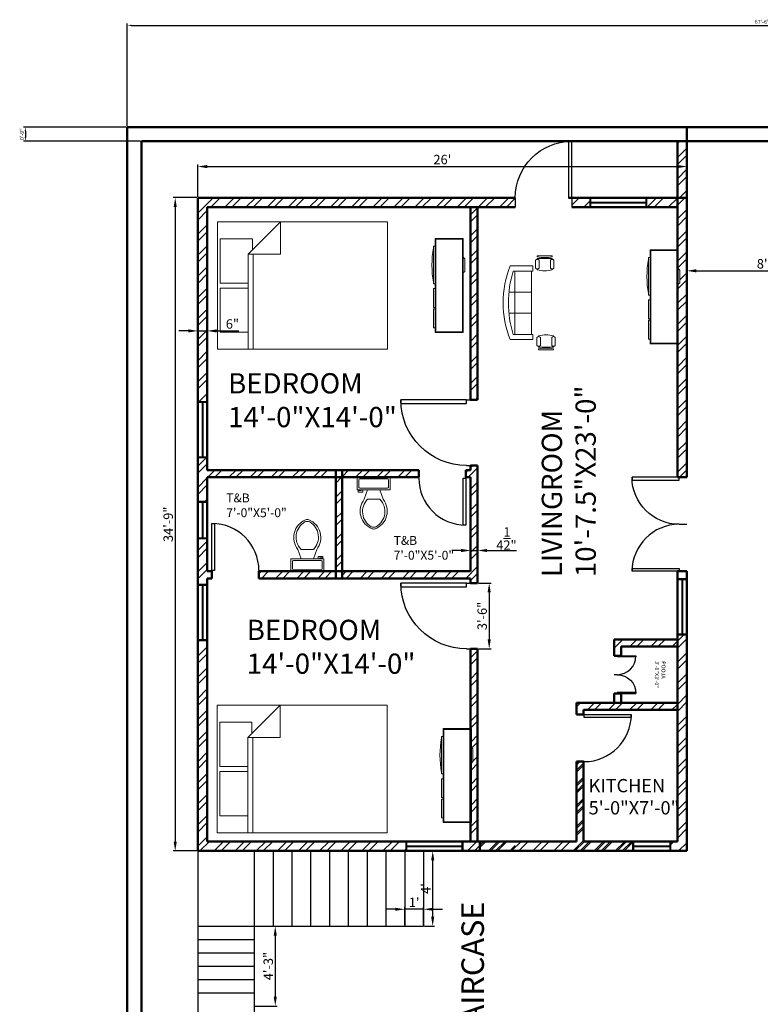
# Model space of a CAD drawing. Units: inches. Extents: x -12550 to 6516, y 1273 to 18700.
# Tile 18 of 19: x 5571 to 6043, y 1958 to 2587. Entities that reach past the tile are written whole.
import ezdxf

# ---------------------------------------------------------------- set-up
doc = ezdxf.new("R2010")
doc.units = ezdxf.units.IN
for name, color, linetype, lineweight in [('A-ANNO-DIMS', 2, 'Continuous', 18), ('A-AREA-IDEN', 1, 'Continuous', 18), ('A-DOOR', 5, 'Continuous', 25), ('A-FLOR-STRS', 6, 'Continuous', 25), ('A-FURN', 8, 'Continuous', 18), ('A-GLAZ', 3, 'Continuous', 25), ('A-WALL', 7, 'Continuous', 50), ('A-WALL-PATT', 8, 'Continuous', 13)]:
    doc.layers.add(name, color=color, linetype=linetype, lineweight=lineweight)
doc.styles.get("Standard").update_dxf_attribs({"font": 'arial.ttf'})
doc.dimstyles.new('ISO-25', dxfattribs={"dimtxt": 2.5, "dimasz": 2.5, "dimexe": 1.25, "dimexo": 0.625, "dimtad": 1, "dimlunit": 4, "dimtxsty": 'Standard', "dimcen": 2.5, "dimadec": 0, "dimazin": 0, "dimtfac": 1, "dimtmove": 0, "dimatfit": 3, "dimfxl": 1, "dimarcsym": 0})
pattern_1 = [(45, (3666.851, 0), (-6.735192, 6.735192), []), (45, (3671.341, 0), (-6.735192, 6.735192), [])]
pattern_2 = [(45, (3666.851, 567), (-6.735192, 6.735192), []), (45, (3671.341, 567), (-6.735192, 6.735192), [])]

# ---------------------------------------------------------------- blocks, each defined once
blk = doc.blocks.new('*U2')
for p, q in [((0, 0), (0, -5)), ((30, 0), (30, -5))]:
    blk.add_line(p, q)
blk.add_lwpolyline([(0, 0), (0, 30), (1.75, 30), (1.75, 0)], close=True)
blk.add_arc((0, 0), 30, 0, 90)
blk = doc.blocks.new('Bed - Queen')
for p, q in [((0, -80.00003), (0, 0)), ((0, 0), (59.99999, 0)), ((59.99999, 0), (59.99999, -80.00003)), ((7.99999, -1.2), (28.79998, -1.2)), ((7.99999, -14.4), (7.99999, -1.2)), ((28.79998, -1.2), (28.79998, -14.4)), ((31.19999, -1.2), (51.99999, -1.2)), ((31.19999, -14.4), (31.19999, -1.2)), ((51.99999, -1.2), (51.99999, -16.4)), ((0, -14.4), (44.8, -14.4)), ((44.8, -16.8), (0, -16.8)), ((59.99999, -29.6), (44.8, -14.4)), ((44.8, -14.4), (44.8, -29.6)), ((51.99999, -16.4), (46.79936, -16.4)), ((44.8, -29.6), (59.99999, -29.6)), ((59.99999, -80.00003), (0, -80.00003))]:
    blk.add_line(p, q)
blk = doc.blocks.new('Toilet - top')
for p, q in [((9.5, -6), (9.5, -2)), ((-10, -8.5), (-8, -8.5)), ((-10, -9.5), (-10, -8.5)), ((-7, -9.5), (-10, -9.5)), ((-8, -8.5), (-8, -8)), ((-7, -8), (-7, -9.5)), ((-4, -8), (-6, -14)), ((4, -8), (6, -14)), ((4, -14), (-4, -14))]:
    blk.add_line(p, q)
blk.add_lwpolyline([(10.5, -8), (10.5, 0), (-10.5, 0), (-10.5, -8)], close=True)
for points in [[(-9.5, -2), (-9.5, -6)], [(8.5, -1), (-8.5, -1)], [(-8.5, -7), (8.5, -7)]]:
    blk.add_lwpolyline(points)
for centre, radius, start, end in [((-8.62, -1.88), 0.884, 81.8699, 188.1301), ((-8.62, -6.12), 0.884, 171.8699, 278.1301), ((8.62, -1.88), 0.884, 351.8699, 98.1301), ((8.62, -6.12), 0.884, 261.8699, 8.1301), ((3.52, -21.58), 12.17, 141.46911, 247.97143), ((4.2, -21.82), 11.33, 136.36773, 238.94682), ((-3.52, -21.58), 12.17, 292.02843, 38.53071), ((-4.2, -21.82), 11.33, 301.05301, 43.63209), ((0, -27.88), 4, 245.73182, 294.26817), ((0, -29), 4, 254.86053, 285.13947)]:
    blk.add_arc(centre, radius, start, end)
blk = doc.blocks.new('Entertainment Center')
for p, q in [((-4, 0), (-5, -1)), ((4, 0), (-4, 0)), ((5, -1), (4, 0)), ((-17, -19), (-17, -1)), ((-17, -1), (43, -1)), ((-16.5, -18.5), (-16.5, -1.5)), ((-16.5, -1.5), (42.5, -1.5)), ((42.5, -1.5), (42.5, -18.5)), ((43, -1), (43, -19)), ((42.5, -18.5), (-16.5, -18.5)), ((43, -19), (-17, -19)), ((-12, -20), (-12, -19)), ((12, -20), (-12, -20)), ((12, -19), (12, -20)), ((15, -20), (15, -19)), ((27, -20), (15, -20)), ((27, -19), (27, -20)), ((28, -20), (28, -19)), ((40, -20), (28, -20)), ((40, -19), (40, -20))]:
    blk.add_line(p, q)
blk.add_arc((0, 40), 61, 259.6111, 280.3889)
blk = doc.blocks.new('Sofa - Roundback 7 ft.')
for p, q in [((-12.00002, -32.4421), (-12.00003, -6.5971)), ((11.99997, -32.4421), (11.99998, -6.5971)), ((-36.000027, -34), (-36.000027, -11.4696)), ((-35.999844, -13.3819), (35.9998, -13.3819)), ((35.99998, -34), (35.99998, -11.4696)), ((-36.000027, -32.4421), (35.99998, -32.4421))]:
    blk.add_line(p, q)
for points in [[(-36.000027, -34), (-42.000027, -34), (-42.000027, -8)], [(41.99998, -8), (41.99998, -34), (35.99998, -34)]]:
    blk.add_lwpolyline(points)
for centre, radius, start, end in [((0, -114.25), 114.25, 68.43141, 111.5686), ((-0.00001, -127.1968), 121.1968, 72.72033, 107.2797)]:
    blk.add_arc(centre, radius, start, end)
blk = doc.blocks.new('Chair - Desk')
for p, q in [((-8.5, 0), (-8.5, -1)), ((-8.5, 0), (8.5, 0)), ((8.5, 0), (8.5, -1)), ((-10.5, -5), (-10.5, -14)), ((-8.5, -3), (-8.5, -4)), ((-8.5, -3), (8.5, -3)), ((-6.5, -14), (-6.5, -5)), ((-2, -3), (-2, -1.9355)), ((2, -1.9576), (2, -3)), ((6.5, -5), (6.5, -14)), ((8.5, -3), (8.5, -4)), ((10.5, -14), (10.5, -5)), ((-8.5, -15), (-8.5, -16)), ((8.5, -15), (8.5, -16))]:
    blk.add_line(p, q)
for centre, radius, start, end in [((-8.5, -6.5), 2.5, 36.8699, 143.1301), ((0, 34.625), 36.625, 256.5803, 283.4197), ((8.5, -6.5), 2.5, 36.8699, 143.1301), ((-8.5, -12.5), 2.5, 216.8699, 323.1301), ((0, 19.625), 36.625, 256.5803, 283.4197), ((8.5, -12.5), 2.5, 216.8699, 323.1301)]:
    blk.add_arc(centre, radius, start, end)
blk = doc.blocks.new('*D49')
at = {"layer": 'A-ANNO-DIMS', "color": 0, "lineweight": -2, "transparency": 16777216}
for p, q in [((5684.54, 2388.03), (5684.54, 2389.43)), ((5690.54, 2388.03), (5690.54, 2389.43)), ((5678.54, 2388.18), (5672.54, 2388.18)), ((5684.54, 2388.18), (5690.54, 2388.18)), ((5696.54, 2388.18), (5710.72, 2388.18))]:
    blk.add_line(p, q, dxfattribs=at)
at = {"layer": 'A-ANNO-DIMS', "color": 0, "transparency": 16777216}
for points in [[(5678.54, 2389.18), (5678.54, 2387.18), (5684.54, 2388.18)], [(5696.54, 2389.18), (5696.54, 2387.18), (5690.54, 2388.18)]]:
    blk.add_solid(points, dxfattribs=at)
at = {"layer": 'Defpoints', "color": 0, "transparency": 16777216}
for p in [(5684.54, 2387.4), (5690.54, 2388.18), (5690.54, 2387.4)]:
    blk.add_point(p, dxfattribs=at)
at = {"layer": 'A-ANNO-DIMS', "color": 0, "transparency": 16777216, "insert": (5706.63, 2391.87), "char_height": 6, "attachment_point": 5}
blk.add_mtext('6"', dxfattribs=at)
blk = doc.blocks.new('*D50')
at = {"layer": 'A-ANNO-DIMS', "color": 0, "lineweight": -2, "transparency": 16777216}
for p, q in [((5858.54, 2251.78), (5858.54, 2246.78)), ((5863.04, 2251.78), (5863.04, 2246.78)), ((5852.54, 2248.03), (5846.54, 2248.03)), ((5858.54, 2248.03), (5863.04, 2248.03)), ((5869.04, 2248.03), (5887.8, 2248.03))]:
    blk.add_line(p, q, dxfattribs=at)
at = {"layer": 'A-ANNO-DIMS', "color": 0, "transparency": 16777216}
for points in [[(5852.54, 2249.03), (5852.54, 2247.03), (5858.54, 2248.03)], [(5869.04, 2249.03), (5869.04, 2247.03), (5863.04, 2248.03)]]:
    blk.add_solid(points, dxfattribs=at)
at = {"layer": 'Defpoints', "color": 0, "transparency": 16777216}
for p in [(5858.54, 2252.41), (5863.04, 2252.41), (5863.04, 2248.03)]:
    blk.add_point(p, dxfattribs=at)
at = {"layer": 'A-ANNO-DIMS', "color": 0, "transparency": 16777216, "insert": (5881.42, 2255.68), "char_height": 6, "attachment_point": 5}
blk.add_mtext('4{\\H1x;\\S1/2;}"', dxfattribs=at)
blk = doc.blocks.new('*D57')
at = {"layer": 'A-ANNO-DIMS', "color": 0, "lineweight": -2, "transparency": 16777216}
for p, q in [((5863.66, 2227.25), (5871.67, 2227.25)), ((5870.42, 2221.25), (5870.42, 2191.25)), ((5863.66, 2185.25), (5871.67, 2185.25))]:
    blk.add_line(p, q, dxfattribs=at)
at = {"layer": 'A-ANNO-DIMS', "color": 0, "transparency": 16777216}
for points in [[(5869.42, 2221.25), (5871.42, 2221.25), (5870.42, 2227.25)], [(5869.42, 2191.25), (5871.42, 2191.25), (5870.42, 2185.25)]]:
    blk.add_solid(points, dxfattribs=at)
at = {"layer": 'Defpoints', "color": 0, "transparency": 16777216}
for p in [(5863.04, 2227.25), (5863.04, 2185.25), (5870.42, 2185.25)]:
    blk.add_point(p, dxfattribs=at)
at = {"layer": 'A-ANNO-DIMS', "color": 0, "transparency": 16777216, "insert": (5866.73, 2206.25), "char_height": 6, "attachment_point": 5, "rotation": 90}
blk.add_mtext('3\'-6"', dxfattribs=at)
blk = doc.blocks.new('*D58')
at = {"layer": 'A-ANNO-DIMS', "color": 0, "lineweight": -2, "transparency": 16777216}
for p, q in [((5829.16, 2056.25), (5835.64, 2056.25)), ((5834.39, 2014.25), (5834.39, 2050.25)), ((5829.16, 2008.25), (5835.64, 2008.25))]:
    blk.add_line(p, q, dxfattribs=at)
at = {"layer": 'A-ANNO-DIMS', "color": 0, "transparency": 16777216}
for points in [[(5833.39, 2050.25), (5835.39, 2050.25), (5834.39, 2056.25)], [(5833.39, 2014.25), (5835.39, 2014.25), (5834.39, 2008.25)]]:
    blk.add_solid(points, dxfattribs=at)
at = {"layer": 'Defpoints', "color": 0, "transparency": 16777216}
for p in [(5828.54, 2056.25), (5834.39, 2056.25), (5828.54, 2008.25)]:
    blk.add_point(p, dxfattribs=at)
at = {"layer": 'A-ANNO-DIMS', "color": 0, "transparency": 16777216, "insert": (5830.77, 2032.25), "char_height": 6, "attachment_point": 5, "rotation": 90}
blk.add_mtext("4'", dxfattribs=at)
blk = doc.blocks.new('*D59')
at = {"layer": 'A-ANNO-DIMS', "color": 0, "lineweight": -2, "transparency": 16777216}
for p, q in [((5810.54, 2019.01), (5804.54, 2019.01)), ((5816.54, 2008.87), (5816.54, 2020.26)), ((5828.54, 2019.01), (5816.54, 2019.01)), ((5828.54, 2008.87), (5828.54, 2020.26)), ((5834.54, 2019.01), (5840.54, 2019.01))]:
    blk.add_line(p, q, dxfattribs=at)
at = {"layer": 'A-ANNO-DIMS', "color": 0, "transparency": 16777216}
for points in [[(5810.54, 2020.01), (5810.54, 2018.01), (5816.54, 2019.01)], [(5834.54, 2020.01), (5834.54, 2018.01), (5828.54, 2019.01)]]:
    blk.add_solid(points, dxfattribs=at)
at = {"layer": 'Defpoints', "color": 0, "transparency": 16777216}
for p in [(5816.54, 2019.01), (5816.54, 2008.25), (5828.54, 2008.25)]:
    blk.add_point(p, dxfattribs=at)
at = {"layer": 'A-ANNO-DIMS', "color": 0, "transparency": 16777216, "insert": (5822.54, 2022.65), "char_height": 6, "attachment_point": 5}
blk.add_mtext("1'", dxfattribs=at)
blk = doc.blocks.new('*D60')
at = {"layer": 'A-ANNO-DIMS', "color": 0, "lineweight": -2, "transparency": 16777216}
for p, q in [((5721.16, 2008.25), (5735.21, 2008.25)), ((5733.96, 2002.25), (5733.96, 1963.25)), ((5721.16, 1957.25), (5735.21, 1957.25))]:
    blk.add_line(p, q, dxfattribs=at)
at = {"layer": 'A-ANNO-DIMS', "color": 0, "transparency": 16777216}
for points in [[(5732.96, 2002.25), (5734.96, 2002.25), (5733.96, 2008.25)], [(5732.96, 1963.25), (5734.96, 1963.25), (5733.96, 1957.25)]]:
    blk.add_solid(points, dxfattribs=at)
at = {"layer": 'Defpoints', "color": 0, "transparency": 16777216}
for p in [(5720.54, 2008.25), (5720.54, 1957.25), (5733.96, 1957.25)]:
    blk.add_point(p, dxfattribs=at)
at = {"layer": 'A-ANNO-DIMS', "color": 0, "transparency": 16777216, "insert": (5730.27, 1982.75), "char_height": 6, "attachment_point": 5, "rotation": 90}
blk.add_mtext('4\'-3"', dxfattribs=at)
blk = doc.blocks.new('*D53')
at = {"layer": 'A-ANNO-DIMS', "color": 0, "lineweight": -2, "transparency": 16777216}
for p, q in [((5683.91, 2473.25), (5668.88, 2473.25)), ((5670.13, 2467.25), (5670.13, 2062.25)), ((5683.91, 2056.25), (5668.88, 2056.25))]:
    blk.add_line(p, q, dxfattribs=at)
at = {"layer": 'A-ANNO-DIMS', "color": 0, "transparency": 16777216}
for points in [[(5669.13, 2467.25), (5671.13, 2467.25), (5670.13, 2473.25)], [(5669.13, 2062.25), (5671.13, 2062.25), (5670.13, 2056.25)]]:
    blk.add_solid(points, dxfattribs=at)
at = {"layer": 'Defpoints', "color": 0, "transparency": 16777216}
for p in [(5684.54, 2473.25), (5670.13, 2056.25), (5684.54, 2056.25)]:
    blk.add_point(p, dxfattribs=at)
at = {"layer": 'A-ANNO-DIMS', "color": 0, "transparency": 16777216, "insert": (5666.44, 2264.75), "char_height": 6, "attachment_point": 5, "rotation": 90}
blk.add_mtext('34\'-9"', dxfattribs=at)
blk = doc.blocks.new('*D56')
at = {"layer": 'A-ANNO-DIMS', "color": 0, "lineweight": -2, "transparency": 16777216}
for p, q in [((5684.54, 2473.87), (5684.54, 2494.36)), ((5690.54, 2493.11), (5990.54, 2493.11)), ((5996.54, 2473.87), (5996.54, 2494.36))]:
    blk.add_line(p, q, dxfattribs=at)
at = {"layer": 'A-ANNO-DIMS', "color": 0, "transparency": 16777216}
for points in [[(5690.54, 2494.11), (5690.54, 2492.11), (5684.54, 2493.11)], [(5990.54, 2494.11), (5990.54, 2492.11), (5996.54, 2493.11)]]:
    blk.add_solid(points, dxfattribs=at)
at = {"layer": 'Defpoints', "color": 0, "transparency": 16777216}
for p in [(5996.54, 2493.11), (5684.54, 2473.25), (5996.54, 2473.25)]:
    blk.add_point(p, dxfattribs=at)
at = {"layer": 'A-ANNO-DIMS', "color": 0, "transparency": 16777216, "insert": (5840.54, 2496.8), "char_height": 6, "attachment_point": 5}
blk.add_mtext("26'", dxfattribs=at)
blk = doc.blocks.new('*D51')
at = {"layer": 'A-ANNO-DIMS', "color": 0, "lineweight": -2, "transparency": 16777216}
for p, q in [((5996.54, 2407.12), (5996.54, 2427.81)), ((6002.54, 2426.56), (6086.54, 2426.56)), ((6092.54, 2407.12), (6092.54, 2427.81))]:
    blk.add_line(p, q, dxfattribs=at)
at = {"layer": 'A-ANNO-DIMS', "color": 0, "transparency": 16777216}
for points in [[(6002.54, 2427.56), (6002.54, 2425.56), (5996.54, 2426.56)], [(6086.54, 2427.56), (6086.54, 2425.56), (6092.54, 2426.56)]]:
    blk.add_solid(points, dxfattribs=at)
at = {"layer": 'Defpoints', "color": 0, "transparency": 16777216}
for p in [(6092.54, 2426.56), (5996.54, 2406.5), (6092.54, 2406.5)]:
    blk.add_point(p, dxfattribs=at)
at = {"layer": 'A-ANNO-DIMS', "color": 0, "transparency": 16777216, "insert": (6044.54, 2430.25), "char_height": 6, "attachment_point": 5}
blk.add_mtext("8'", dxfattribs=at)
blk = doc.blocks.new('WIN-3FT')
for p, q in [((0, 0), (0, 6)), ((0, 6), (36.02, 6)), ((36.02, 0), (0, 0)), ((0.5, 0), (0.5, 6)), ((35.52, 3.2), (0.5, 3.2)), ((35.52, 2.8), (0.5, 2.8)), ((35.52, 6), (35.52, 0)), ((36.02, 6), (36.02, 0))]:
    blk.add_line(p, q)
blk = doc.blocks.new('WIN-2FT')
for p, q in [((0, 0), (0, 24.02)), ((0, 24.02), (6, 24.02)), ((0, 23.52), (6, 23.52)), ((2.8, 0.5), (2.8, 23.52)), ((3.2, 0.5), (3.2, 23.52)), ((6, 24.02), (6, 0)), ((6, 0.5), (0, 0.5)), ((6, 0), (0, 0))]:
    blk.add_line(p, q)
blk = doc.blocks.new('*D121')
at = {"layer": 'A-ANNO-DIMS', "color": 0, "lineweight": -2, "transparency": 16777216}
for p, q in [((5639.54, 2518.87), (5639.54, 2584.5)), ((5642.04, 2583.25), (6447.04, 2583.25)), ((6449.54, 2518.87), (6449.54, 2584.5))]:
    blk.add_line(p, q, dxfattribs=at)
at = {"layer": 'A-ANNO-DIMS', "color": 0, "transparency": 16777216}
for points in [[(5642.04, 2583.66), (5642.04, 2582.83), (5639.54, 2583.25)], [(6447.04, 2583.66), (6447.04, 2582.83), (6449.54, 2583.25)]]:
    blk.add_solid(points, dxfattribs=at)
at = {"layer": 'Defpoints', "color": 0, "transparency": 16777216}
for p in [(6449.54, 2583.25), (5639.54, 2518.25), (6449.54, 2518.25)]:
    blk.add_point(p, dxfattribs=at)
at = {"layer": 'A-ANNO-DIMS', "color": 0, "transparency": 16777216, "insert": (6044.54, 2585.15), "char_height": 2.5, "attachment_point": 5}
blk.add_mtext('67\'-6"', dxfattribs=at)
blk = doc.blocks.new('*D129')
at = {"layer": 'A-ANNO-DIMS', "color": 0, "lineweight": -2, "transparency": 16777216}
for p, q in [((5638.91, 2518.25), (5573.29, 2518.25)), ((5574.54, 2515.75), (5574.54, 2511.75)), ((5647.91, 2509.25), (5573.29, 2509.25))]:
    blk.add_line(p, q, dxfattribs=at)
at = {"layer": 'A-ANNO-DIMS', "color": 0, "transparency": 16777216}
for points in [[(5574.12, 2515.75), (5574.96, 2515.75), (5574.54, 2518.25)], [(5574.12, 2511.75), (5574.96, 2511.75), (5574.54, 2509.25)]]:
    blk.add_solid(points, dxfattribs=at)
at = {"layer": 'Defpoints', "color": 0, "transparency": 16777216}
for p in [(5639.54, 2518.25), (5574.54, 2509.25), (5648.54, 2509.25)]:
    blk.add_point(p, dxfattribs=at)
at = {"layer": 'A-ANNO-DIMS', "color": 0, "transparency": 16777216, "insert": (5572.64, 2513.75), "char_height": 2.5, "attachment_point": 5, "rotation": 90}
blk.add_mtext('0\'-9"', dxfattribs=at)

msp = doc.modelspace()

# ---------------------------------------------------------------- hatches: boundary and pattern name
at = {"layer": 'A-WALL-PATT'}
h = msp.add_hatch(dxfattribs=at)
h.set_pattern_fill('ANSI32', color=256)
h.set_pattern_definition(pattern_1)
h.paths.add_polyline_path([(5996.54, 2509.247), (5990.54, 2509.247), (5990.54, 2473.247), (5996.54, 2473.247)])
h = msp.add_hatch(dxfattribs=at)
h.set_pattern_fill('ANSI32', color=256)
h.set_pattern_definition(pattern_2)
h.paths.add_polyline_path([(5690.54, 2467.247), (5864.54, 2467.247), (5864.54, 2473.247), (5684.54, 2473.247), (5684.54, 2343.138), (5690.54, 2343.138)])
h = msp.add_hatch(dxfattribs=at)
h.set_pattern_fill('ANSI32', color=256)
h.set_pattern_definition(pattern_2)
h.paths.add_polyline_path([(5923.04, 2473.247), (5923.04, 2467.247), (5934.791, 2467.247), (5934.791, 2473.247)])
h.paths.add_polyline_path([(5887.04, 2467.247), (5887.04, 2473.247), (5864.54, 2473.247), (5864.54, 2467.247)])
h = msp.add_hatch(dxfattribs=at)
h.set_pattern_fill('ANSI32', color=256)
h.set_pattern_definition(pattern_2)
h.paths.add_polyline_path([(5996.54, 2473.247), (5970.808, 2473.247), (5970.808, 2467.247), (5990.54, 2467.247), (5990.54, 2439.972), (5991.04, 2439.972), (5991.04, 2427.972), (5992.04, 2426.972), (5992.04, 2418.972), (5991.04, 2417.972), (5991.04, 2379.972), (5990.54, 2294.747), (5991.54, 2294.747), (5996.54, 2294.747)])
h = msp.add_hatch(dxfattribs=at)
h.set_pattern_fill('ANSI32', color=256)
h.set_pattern_definition(pattern_2)
h.paths.add_polyline_path([(5863.04, 2467.247), (5858.54, 2467.247), (5858.54, 2344.247), (5863.04, 2344.247)], flags=17)
h = msp.add_hatch(dxfattribs=at)
h.set_pattern_fill('ANSI32', color=256)
h.set_pattern_definition(pattern_2)
h.paths.add_polyline_path([(5772.54, 2299.247), (5690.54, 2299.247), (5690.54, 2307.121), (5684.54, 2307.121), (5684.54, 2279.466), (5690.54, 2279.466), (5690.54, 2294.747), (5772.54, 2294.747)])
h = msp.add_hatch(dxfattribs=at)
h.set_pattern_fill('ANSI32', color=256)
h.set_pattern_definition(pattern_2)
h.paths.add_polyline_path([(5863.04, 2302.247), (5858.54, 2302.247), (5858.54, 2299.247), (5855.54, 2299.247), (5855.54, 2294.747), (5858.54, 2294.747), (5858.54, 2234.747), (5776.54, 2234.747), (5776.54, 2230.247), (5858.54, 2230.247), (5858.54, 2227.247), (5863.04, 2227.247)])
h = msp.add_hatch(dxfattribs=at)
h.set_pattern_fill('ANSI32', color=256)
h.set_pattern_definition(pattern_2)
h.paths.add_polyline_path([(5776.54, 2294.747), (5772.54, 2294.747), (5772.54, 2234.747), (5776.54, 2234.747)])
h = msp.add_hatch(dxfattribs=at)
h.set_pattern_fill('ANSI32', color=256)
h.set_pattern_definition(pattern_2)
h.paths.add_polyline_path([(5825.54, 2299.247), (5776.54, 2299.247), (5776.54, 2294.747), (5825.54, 2294.747)], flags=17)
h = msp.add_hatch(dxfattribs=at)
h.set_pattern_fill('ANSI32', color=256)
h.set_pattern_definition(pattern_2)
h.paths.add_polyline_path([(5690.54, 2255.449), (5684.54, 2255.449), (5684.54, 2226.453), (5690.54, 2226.453), (5690.54, 2230.247), (5693.54, 2230.247), (5693.54, 2234.747), (5690.54, 2234.747)])
h = msp.add_hatch(dxfattribs=at)
h.set_pattern_fill('ANSI32', color=256)
h.set_pattern_definition(pattern_2)
h.paths.add_polyline_path([(5772.54, 2234.747), (5723.54, 2234.747), (5723.54, 2230.247), (5772.54, 2230.247)])
h = msp.add_hatch(dxfattribs=at)
h.set_pattern_fill('ANSI32', color=256)
h.set_pattern_definition(pattern_2)
h.paths.add_polyline_path([(5996.54, 2194.032), (5990.54, 2194.032), (5990.54, 2062.247), (5986.145, 2062.247), (5986.145, 2056.247), (5996.54, 2056.247)])
h = msp.add_hatch(dxfattribs=at)
h.set_pattern_fill('ANSI32', color=256)
h.set_pattern_definition(pattern_2)
h.paths.add_polyline_path([(5690.54, 2190.435), (5684.54, 2190.435), (5684.54, 2056.247), (5817.49, 2056.247), (5817.49, 2062.247), (5690.54, 2062.247)])
h = msp.add_hatch(dxfattribs=at)
h.set_pattern_fill('ANSI32', color=256)
h.set_pattern_definition(pattern_2)
h.paths.add_polyline_path([(5990.54, 2191.247), (5950.04, 2191.247), (5950.04, 2180.747), (5952.04, 2180.747), (5954.54, 2180.747), (5954.54, 2186.747), (5990.54, 2186.747)])
h = msp.add_hatch(dxfattribs=at)
h.set_pattern_fill('ANSI32', color=256)
h.set_pattern_definition(pattern_2)
h.paths.add_polyline_path([(5863.04, 2185.247), (5858.54, 2185.247), (5858.54, 2134.365), (5859.04, 2134.365), (5859.04, 2122.365), (5860.04, 2121.365), (5860.04, 2113.365), (5859.04, 2112.365), (5859.04, 2074.365), (5858.54, 2062.247), (5863.04, 2062.247)])
h = msp.add_hatch(dxfattribs=at)
h.set_pattern_fill('ANSI32', color=256)
h.set_pattern_definition(pattern_2)
h.paths.add_polyline_path([(5990.54, 2150.747), (5926.04, 2150.747), (5926.04, 2143.247), (5930.54, 2143.247), (5930.54, 2146.247), (5990.54, 2146.247)])
h = msp.add_hatch(dxfattribs=at)
h.set_pattern_fill('ANSI32', color=256)
h.set_pattern_definition(pattern_1)
h.paths.add_polyline_path([(5962.127, 2062.247), (5930.54, 2062.247), (5930.54, 2113.247), (5926.04, 2113.247), (5926.04, 2062.247), (5923.04, 2062.247), (5864.54, 2062.247), (5864.54, 2056.247), (5923.04, 2056.247), (5962.127, 2056.247)])
h = msp.add_hatch(dxfattribs=at)
h.set_pattern_fill('ANSI32', color=256)
h.set_pattern_definition(pattern_2)
h.paths.add_polyline_path([(5930.54, 2062.247), (5930.54, 2113.247), (5926.04, 2113.247), (5926.04, 2062.247), (5923.04, 2062.247), (5923.04, 2056.247), (5962.127, 2056.247), (5962.127, 2062.247)])
h = msp.add_hatch(dxfattribs=at)
h.set_pattern_fill('ANSI32', color=256)
h.set_pattern_definition(pattern_2)
h.paths.add_polyline_path([(5853.508, 2062.247), (5853.508, 2056.247), (5887.04, 2056.247), (5887.04, 2062.247)])

# ---------------------------------------------------------------- linework, layer by layer
at = {"layer": 'A-FLOR-STRS'}
for p, q in [((5864.54, 2056.247), (5684.54, 2056.247)), ((5684.54, 2056.247), (5684.54, 1906.247)), ((5720.54, 2056.247), (5720.54, 1906.247)), ((5732.54, 2056.247), (5732.54, 2008.247)), ((5744.54, 2056.247), (5744.54, 2008.247)), ((5756.54, 2056.247), (5756.54, 2008.247)), ((5768.54, 2056.247), (5768.54, 2008.247)), ((5780.54, 2056.247), (5780.54, 2008.247)), ((5792.54, 2056.247), (5792.54, 2008.247)), ((5804.54, 2056.247), (5804.54, 2008.247)), ((5816.54, 2056.247), (5816.54, 2008.247)), ((5828.54, 2056.247), (5828.54, 2008.247)), ((5684.54, 2008.247), (5828.54, 2008.247)), ((5684.54, 2008.247), (5828.54, 2008.247)), ((5684.54, 1999.747), (5720.54, 1999.747)), ((5684.54, 1991.247), (5720.54, 1991.247)), ((5684.54, 1982.747), (5720.54, 1982.747)), ((5684.54, 1974.247), (5720.54, 1974.247)), ((5684.54, 1965.747), (5720.54, 1965.747))]:
    msp.add_line(p, q, dxfattribs=at)
at = {"layer": 'A-WALL'}
for p, q in [((5639.54, 1444.247), (5639.54, 2518.247)), ((5639.54, 2518.247), (6449.54, 2518.247)), ((5996.54, 2294.747), (5996.54, 2518.247)), ((5648.54, 1453.247), (5648.54, 2509.247)), ((5648.54, 2509.247), (6440.54, 2509.247)), ((6220.94, 2509.247), (5920.94, 2509.247)), ((5990.54, 2294.747), (5990.54, 2509.247)), ((5887.04, 2473.247), (5684.54, 2473.247)), ((5684.54, 2068.324), (5684.54, 2473.247)), ((5996.54, 2473.247), (5920.94, 2473.247)), ((5887.04, 2467.247), (5690.54, 2467.247)), ((5690.54, 2299.247), (5690.54, 2467.247)), ((5858.54, 2344.247), (5858.54, 2467.247)), ((5863.04, 2344.247), (5863.04, 2467.247)), ((5990.54, 2467.247), (5923.04, 2467.247)), ((5863.04, 2344.247), (5858.54, 2344.247)), ((5858.54, 2299.247), (5858.54, 2302.247)), ((5858.54, 2299.247), (5858.54, 2302.247)), ((5858.54, 2302.247), (5863.04, 2302.247)), ((5863.04, 2227.247), (5863.04, 2302.247)), ((5825.54, 2299.247), (5690.54, 2299.247)), ((5825.54, 2294.747), (5690.54, 2294.747)), ((5690.54, 2234.747), (5690.54, 2294.747)), ((5772.54, 2230.247), (5772.54, 2299.247)), ((5776.54, 2230.247), (5776.54, 2299.247)), ((5825.54, 2294.747), (5825.54, 2299.247)), ((5858.54, 2299.247), (5855.54, 2299.247)), ((5858.54, 2299.247), (5855.54, 2299.247)), ((5855.54, 2299.247), (5855.54, 2294.747)), ((5858.54, 2294.747), (5855.54, 2294.747)), ((5858.54, 2234.747), (5858.54, 2294.747)), ((5996.54, 2294.747), (5990.54, 2294.747)), ((5693.54, 2234.747), (5690.54, 2234.747)), ((5693.54, 2230.247), (5693.54, 2234.747)), ((5858.54, 2234.747), (5723.54, 2234.747)), ((5723.54, 2234.747), (5858.54, 2234.747)), ((5723.54, 2234.747), (5723.54, 2230.247)), ((5996.54, 2234.747), (5990.54, 2234.747)), ((5990.54, 2062.247), (5990.54, 2234.747)), ((5996.54, 2056.247), (5996.54, 2234.747)), ((5693.54, 2230.247), (5690.54, 2230.247)), ((5690.54, 2062.247), (5690.54, 2230.247)), ((5690.54, 2230.247), (5693.54, 2230.247)), ((5858.54, 2230.247), (5723.54, 2230.247)), ((5858.54, 2227.247), (5858.54, 2230.247)), ((5863.04, 2227.247), (5858.54, 2227.247)), ((5863.04, 2230.247), (5863.04, 2227.247)), ((5990.54, 2191.247), (5950.04, 2191.247)), ((5950.04, 2180.747), (5950.04, 2191.247)), ((5858.54, 2062.247), (5858.54, 2185.247)), ((5858.54, 2185.247), (5863.04, 2185.247)), ((5863.04, 2062.247), (5863.04, 2185.247)), ((5990.54, 2186.747), (5954.54, 2186.747)), ((5954.54, 2180.747), (5954.54, 2186.747)), ((5950.04, 2180.747), (5954.54, 2180.747)), ((5950.04, 2150.747), (5950.04, 2156.747)), ((5954.54, 2156.747), (5950.04, 2156.747)), ((5954.54, 2150.747), (5954.54, 2156.747)), ((5954.54, 2150.747), (5954.54, 2156.747)), ((5990.54, 2150.747), (5926.04, 2150.747)), ((5926.04, 2143.247), (5926.04, 2150.747)), ((5950.04, 2150.747), (5950.04, 2155.747)), ((5930.54, 2143.247), (5926.04, 2143.247)), ((5990.54, 2146.247), (5930.54, 2146.247)), ((5930.54, 2143.247), (5930.54, 2146.247)), ((5930.54, 2146.247), (5930.54, 2143.247)), ((5926.04, 2062.247), (5926.04, 2113.247)), ((5926.04, 2113.247), (5930.54, 2113.247)), ((5930.54, 2062.247), (5930.54, 2113.247)), ((5684.54, 2056.247), (5684.54, 2068.324)), ((5923.04, 2062.247), (5690.54, 2062.247)), ((5887.04, 2062.247), (5863.04, 2062.247)), ((5864.54, 2056.247), (5864.54, 2062.247)), ((5926.04, 2062.247), (5923.04, 2062.247)), ((5926.04, 2062.247), (5923.04, 2062.247)), ((5990.54, 2062.247), (5930.54, 2062.247)), ((5923.04, 2056.247), (5684.54, 2056.247)), ((5996.54, 2056.247), (5923.04, 2056.247))]:
    msp.add_line(p, q, dxfattribs=at)

# ---------------------------------------------------------------- block references
at = {"layer": 'A-DOOR', "xscale": -1.199999999999999, "yscale": 1.199999999999999, "zscale": 1.199999999999999}
msp.add_blockref('*U2', (5923.04, 2473.247), dxfattribs=at)
at = {"layer": 'A-DOOR'}
for p, xscale, yscale, zscale, rotation in [((5856.04, 2344.247), -1.4, 1.4, 1.4, 90), ((5856.04, 2227.247), -1.4, 1.4, 1.4, 90), ((5952.04, 2180.747), 0.399999999999997, 0.399999999999997, 0.399999999999997, 270), ((5952.04, 2156.747), -0.399999999999997, 0.399999999999997, 0.399999999999997, 270)]:
    msp.add_blockref('*U2', p, dxfattribs=dict(at, xscale=xscale, yscale=yscale, zscale=zscale, rotation=rotation))
for p, rotation in [((5855.54, 2294.247), 180), ((5991.54, 2234.747), 90), ((5931.04, 2143.247), 270)]:
    msp.add_blockref('*U2', p, dxfattribs=dict(at, rotation=rotation))
at = {"layer": 'A-DOOR', "xscale": -1, "rotation": 90}
msp.add_blockref('*U2', (5991.54, 2294.747), dxfattribs=at)
at = {"layer": 'A-DOOR'}
msp.add_blockref('*U2', (5693.54, 2235.247), dxfattribs=at)
at = {"layer": 'A-FURN'}
for name, p, xscale, yscale, zscale, rotation in [('Bed - Queen', (5697.19, 2376.493), 1.354827908062564, 1.354827908062564, 1.354827908062564, 90), ('Sofa - Roundback 7 ft.', (5879.299, 2406.138), 0.5595223685495907, 0.5595223685495907, 0.5595223685495907, 90), ('Chair - Desk', (5906.738, 2376.138), 0.5595223685495907, 0.5595223685495907, 0.5595223685495907, 180), ('Bed - Queen', (5696.888, 2067.915), 1.354827908062564, 1.354827908062564, 1.354827908062564, 90)]:
    msp.add_blockref(name, p, dxfattribs=dict(at, xscale=xscale, yscale=yscale, zscale=zscale, rotation=rotation))
for name, p, rotation in [('Entertainment Center', (5854.881, 2430.204), 270), ('Entertainment Center', (5992.04, 2422.972), 270), ('Toilet - top', (5754.387, 2234.747), 180), ('Entertainment Center', (5860.04, 2117.365), 270)]:
    msp.add_blockref(name, p, dxfattribs=dict(at, rotation=rotation))
at = {"layer": 'A-FURN', "xscale": 0.5595223685495907, "yscale": 0.5595223685495907, "zscale": 0.5595223685495907}
msp.add_blockref('Chair - Desk', (5905.884, 2436.122), dxfattribs=at)
at = {"layer": 'A-FURN'}
msp.add_blockref('Toilet - top', (5796.751, 2294.747), dxfattribs=at)
at = {"layer": 'A-GLAZ'}
for name, p, rotation in [('WIN-3FT', (5970.808, 2473.247), 180), ('WIN-3FT', (5690.54, 2307.121), 90.00000000000468), ('WIN-2FT', (5690.539, 2279.467), 180), ('WIN-3FT', (5690.54, 2190.436), 90.00000000000493), ('WIN-3FT', (5996.54, 2194.032), 89.99999999999908), ('WIN-3FT', (5853.508, 2062.247), 180), ('WIN-2FT', (5962.127, 2062.247), 269.9999999999995)]:
    msp.add_blockref(name, p, dxfattribs=dict(at, rotation=rotation))

# ---------------------------------------------------------------- texts
at = {"layer": 'A-AREA-IDEN', "char_height": 12.93169, "attachment_point": 1}
for insert in [(5703.876, 2361.217), (5715.757, 2203.812)]:
    msp.add_mtext('BEDROOM\\P14\'-0"X14\'-0"', dxfattribs=dict(at, insert=insert))
at = {"layer": 'A-AREA-IDEN', "insert": (5903.946, 2231.034), "char_height": 12.93169, "attachment_point": 1, "rotation": 90}
msp.add_mtext('LIVINGROOM\\P10\'-7.5"X23\'-0"', dxfattribs=at)
at = {"layer": 'A-AREA-IDEN', "attachment_point": 1}
for s, width, gutter_width, insert, char_height in [('T&B\\P7\'-0"X5\'-0"', 4.19569, 28.328, (5702.715, 2284.416), 5.66556), ('T&B\\P7\'-0"X5\'-0"', 4.19569, 28.328, (5809.477, 2257.282), 5.66556), ('KITCHEN\\P5\'-0"X7\'-0"', 1.29487, 42.422, (5933.861, 2102.176), 8.48435)]:
    msp.add_mtext_dynamic_manual_height_columns(s, width=width, gutter_width=gutter_width, heights=[0], dxfattribs=dict(at, insert=insert, char_height=char_height))
for s, width, gutter_width, insert, char_height, rotation in [('POOJA\\P3\'-0"X3\'-0"', 0.78585, 12.5, (5982.916, 2177.304), 2.5, 269.183853), ('STAIRCASE', 2.19144, 71.795, (5852.716, 1922.837), 14.3589, 90)]:
    msp.add_mtext_dynamic_manual_height_columns(s, width=width, gutter_width=gutter_width, heights=[0], dxfattribs=dict(at, insert=insert, char_height=char_height, rotation=rotation))

# ---------------------------------------------------------------- dimensions: what is measured, and where the dimension line sits
at = {"layer": 'A-ANNO-DIMS'}
for base, p1, p2, override, picture, middle in [((6449.54, 2583.247), (5639.54, 2518.247), (6449.54, 2518.247), {"dimdec": 1, "dimlfac": 1, "dimrnd": 0, "dimzin": 1, "dimdsep": 46, "dimlunit": 4, "dimfrac": 2}, '*D121', (6044.54, 2585.149)), ((5996.54, 2493.114), (5684.54, 2473.247), (5996.54, 2473.247), {"dimtxt": 6, "dimasz": 6, "dimclrd": 0, "dimclre": 0, "dimclrt": 0}, '*D56', (5840.54, 2496.802)), ((6092.54, 2426.562), (5996.54, 2406.497), (6092.54, 2406.497), {"dimtxt": 6, "dimasz": 6, "dimclrd": 0, "dimclre": 0, "dimclrt": 0}, '*D51', (6044.54, 2430.25)), ((5690.54, 2388.182), (5684.54, 2387.405), (5690.54, 2387.405), {"dimtxt": 6, "dimasz": 6, "dimclrd": 0, "dimclre": 0, "dimclrt": 0}, '*D49', (5706.629, 2391.871)), ((5863.04, 2248.034), (5858.54, 2252.406), (5863.04, 2252.406), {"dimtxt": 6, "dimasz": 6, "dimclrd": 0, "dimclre": 0, "dimclrt": 0}, '*D50', (5881.421, 2255.683)), ((5816.54, 2019.012), (5828.54, 2008.247), (5816.54, 2008.247), {"dimtxt": 6, "dimasz": 6, "dimclrd": 0, "dimclre": 0, "dimclrt": 0}, '*D59', (5822.54, 2022.65))]:
    dim = msp.add_linear_dim(base=base, p1=p1, p2=p2, dimstyle='ISO-25', override=override, dxfattribs=at)
    dim.commit()
    dim.dimension.update_dxf_attribs({"geometry": picture, "text_midpoint": middle})
for base, p1, p2, override, picture, middle in [((5574.54, 2509.247), (5639.54, 2518.247), (5648.54, 2509.247), {"dimdec": 1, "dimlfac": 1, "dimrnd": 0, "dimzin": 1, "dimdsep": 46, "dimlunit": 4, "dimfrac": 2}, '*D129', (5572.638, 2513.747)), ((5670.131, 2056.247), (5684.54, 2473.247), (5684.54, 2056.247), {"dimtxt": 6, "dimasz": 6, "dimclrd": 0, "dimclre": 0, "dimclrt": 0}, '*D53', (5666.441, 2264.747)), ((5870.423, 2185.247), (5863.04, 2227.247), (5863.04, 2185.247), {"dimtxt": 6, "dimasz": 6, "dimclrd": 0, "dimclre": 0, "dimclrt": 0}, '*D57', (5866.732, 2206.247)), ((5834.392, 2056.247), (5828.54, 2008.247), (5828.54, 2056.247), {"dimtxt": 6, "dimasz": 6, "dimclrd": 0, "dimclre": 0, "dimclrt": 0}, '*D58', (5830.767, 2032.247)), ((5733.962, 1957.247), (5720.54, 2008.247), (5720.54, 1957.247), {"dimtxt": 6, "dimasz": 6, "dimclrd": 0, "dimclre": 0, "dimclrt": 0}, '*D60', (5730.271, 1982.747))]:
    dim = msp.add_linear_dim(base=base, p1=p1, p2=p2, angle=90, dimstyle='ISO-25', override=override, dxfattribs=at)
    dim.commit()
    dim.dimension.update_dxf_attribs({"geometry": picture, "text_midpoint": middle})

doc.saveas('drawing.dxf')
